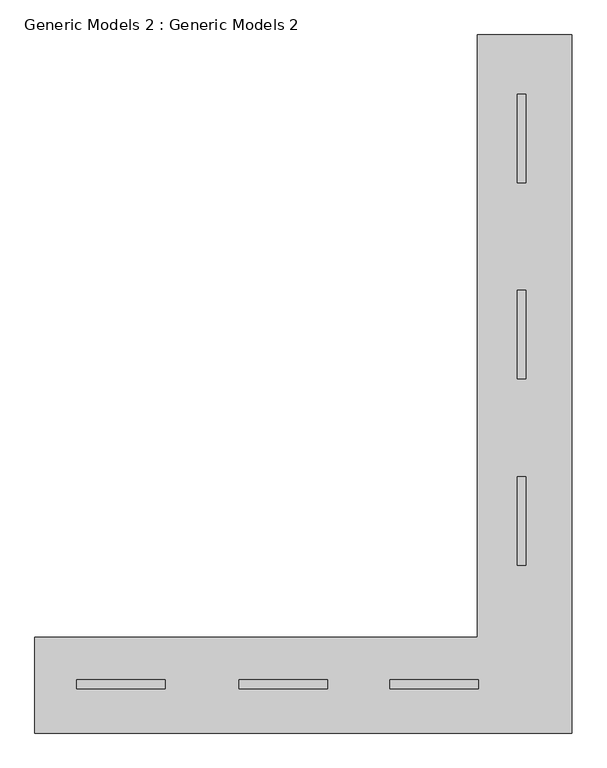
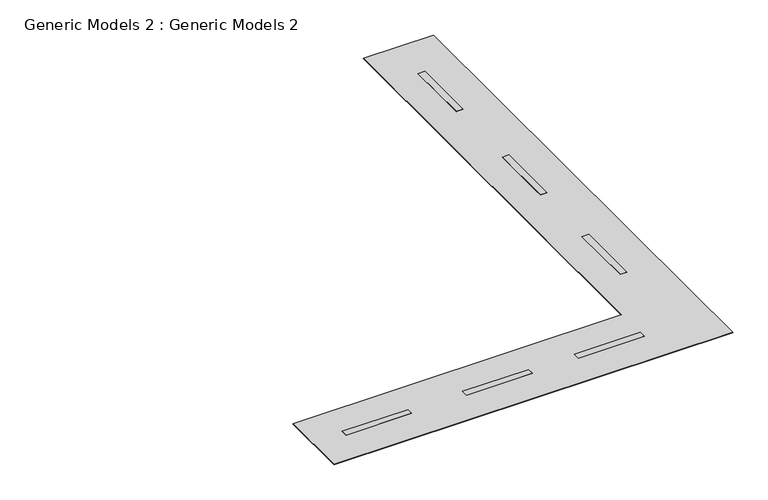
"""IFC4 building model written with IfcOpenShell, lengths in millimetres: proxy geometry, Generic Models 2 : Generic Models 2."""

from ifc_helpers import new_model, si_unit, frame, origin, place, context, project, spatial, polyline, outline, extrude, source, transform, mapped, element, save


def generic_models_2_generic_models_2_e2c80ef7(model_context):
    return source(origin(), model_context, "Body", "SweptSolid", [
        extrude(outline(polyline([(-11829.8744544, -16009.7627865), (-11829.8744544, -15552.5627865), (-7257.8744544, -15552.5627865), (-7257.8744544, -16009.7627865), (-11829.8744544, -16009.7627865)])), frame((0.0, 0.0, -127.0), z_axis=(0.0, 0.0, 1.0), x_axis=(1.0, 0.0, 0.0)), (0.0, 0.0, 1.0), 12.7),
        extrude(outline(polyline([(-3447.8744544, -16009.7627865), (-3447.8744544, -15552.5627865), (1124.1255456, -15552.5627865), (1124.1255456, -16009.7627865), (-3447.8744544, -16009.7627865)])), frame((0.0, 0.0, -127.0), z_axis=(0.0, 0.0, 1.0), x_axis=(1.0, 0.0, 0.0)), (0.0, 0.0, 1.0), 12.7),
        extrude(outline(polyline([(4324.5255456, -16009.7627865), (4324.5255456, -15552.5627865), (8896.5255456, -15552.5627865), (8896.5255456, -16009.7627865), (4324.5255456, -16009.7627865)])), frame((0.0, 0.0, -127.0), z_axis=(0.0, 0.0, 1.0), x_axis=(1.0, 0.0, 0.0)), (0.0, 0.0, 1.0), 12.7),
        extrude(outline(polyline([(11348.4418298, -9662.6325219), (10891.2418298, -9662.6325219), (10891.2418298, -5090.6325219), (11348.4418298, -5090.6325219), (11348.4418298, -9662.6325219)])), frame((0.0, 0.0, -127.0), z_axis=(0.0, 0.0, 1.0), x_axis=(1.0, 0.0, 0.0)), (0.0, 0.0, 1.0), 12.7),
        extrude(outline(polyline([(11348.4418298, -50.1846737), (10891.2418298, -50.1846737), (10891.2418298, 4521.8153263), (11348.4418298, 4521.8153263), (11348.4418298, -50.1846737)])), frame((0.0, 0.0, -127.0), z_axis=(0.0, 0.0, 1.0), x_axis=(1.0, 0.0, 0.0)), (0.0, 0.0, 1.0), 12.7),
        extrude(outline(polyline([(11348.4418298, 10058.8153263), (10891.2418298, 10058.8153263), (10891.2418298, 14630.8153263), (11348.4418298, 14630.8153263), (11348.4418298, 10058.8153263)])), frame((0.0, 0.0, -127.0), z_axis=(0.0, 0.0, 1.0), x_axis=(1.0, 0.0, 0.0)), (0.0, 0.0, 1.0), 12.7),
        extrude(outline(polyline([(8843.6710959, -13371.1881636), (8843.6710959, 17678.8153263), (13720.4710959, 17678.8153263), (13720.4710959, -13371.1881636), (13720.4710959, -18299.3138913), (-13978.2289041, -18299.3138913), (-13978.2289041, -13371.1881636), (8843.6710959, -13371.1881636)])), frame((0.0, 0.0, -152.4), z_axis=(0.0, 0.0, 1.0), x_axis=(1.0, 0.0, 0.0)), (0.0, 0.0, 1.0), 25.4),
    ])


if __name__ == "__main__":
    model = new_model("IFC4")
    model_context = context("Model", 3, world=origin())
    ifc_project = project(units=[si_unit("LENGTHUNIT", "METRE", prefix="MILLI")], contexts=[model_context])
    site = spatial("IfcSite", under=ifc_project)
    building = spatial("IfcBuilding", under=site)
    placement = place(None, origin())
    generic_models_2_generic_models_2_shape = generic_models_2_generic_models_2_e2c80ef7(model_context)
    element("IfcBuildingElementProxy", 1, Name="Generic Models 2 : Generic Models 2", ObjectType="Generic Models 2 : Generic Models 2", at=placement, inside=building, context=model_context, shape_type="MappedRepresentation", body=[
        mapped(generic_models_2_generic_models_2_shape, transform((0.0, 0.0, 0.0), x_axis=(1.0, 0.0, 0.0), y_axis=(0.0, 1.0, 0.0), z_axis=(0.0, 0.0, 1.0))),
    ])
    save(model, "model.ifc")

# Revit data of these elements
# Element 1 (IfcBuildingElementProxy, "Generic Models 2 : Generic Models 2")
#   Materials on its faces: "road"
# Materials
#   "road": class "Generic", colour RGB 0 0 0, transparency 0, Cost = 0
